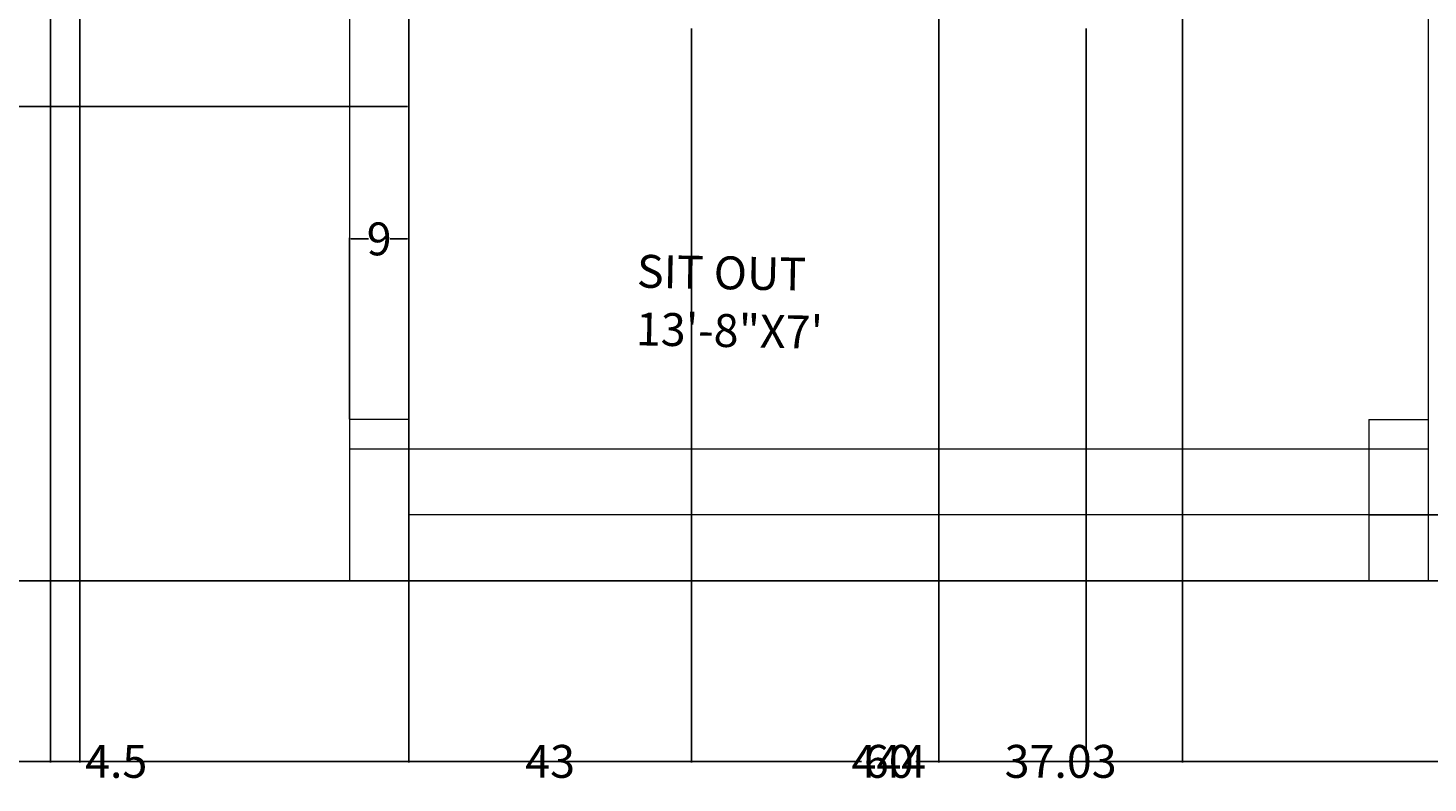
# Model space of a CAD drawing. Units: inches. Extents: x 2807 to 3326, y 2005 to 2580.
# Tile 2 of 12: x 2936 to 3149, y 2005 to 2120. Entities that reach past the tile are written whole.
import ezdxf

# ---------------------------------------------------------------- set-up
doc = ezdxf.new("R2010")
doc.units = ezdxf.units.IN
doc.header["$LTSCALE"] = 0.4
for name, color, linetype, lineweight in [('A-ANNO-DIMS', 2, 'Continuous', 18), ('A-AREA-IDEN', 5, 'Continuous', 18), ('A-FLOR-STRS', 233, 'Continuous', 18)]:
    doc.layers.add(name, color=color, linetype=linetype, lineweight=lineweight)
doc.styles.get("Standard").update_dxf_attribs({"font": 'txt', "height": 5})
doc.dimstyles.get("Standard").update_dxf_attribs({"dimtxt": 0.18, "dimasz": 0.18, "dimexe": 0.18, "dimexo": 0.0625, "dimgap": 0.09, "dimtad": 0, "dimtih": 1, "dimtoh": 1, "dimdec": 4, "dimzin": 0, "dimdsep": 46, "dimtxsty": 'Standard', "dimcen": 0.09, "dimadec": 0, "dimazin": 0, "dimtfac": 1, "dimtdec": 4, "dimtofl": 0, "dimtmove": 0, "dimatfit": 3, "dimfxl": 1, "dimtolj": 1, "dimtzin": 0, "dimarcsym": 0})

# ---------------------------------------------------------------- blocks, each defined once
blk = doc.blocks.new('*D31')
at = {"layer": 'A-ANNO-DIMS', "color": 0, "lineweight": -2, "ltscale": 0.4, "transparency": 16777216}
for p, q in [((2844.57, 2135.51), (2844.57, 2008.45)), ((3288.57, 2135.51), (3288.57, 2008.45)), ((2844.75, 2008.63), (3059.93, 2008.63)), ((3288.39, 2008.63), (3073.2, 2008.63))]:
    blk.add_line(p, q, dxfattribs=at)
at = {"layer": 'A-ANNO-DIMS', "color": 0, "ltscale": 0.4, "transparency": 16777216}
for points in [[(2844.75, 2008.66), (2844.75, 2008.6), (2844.57, 2008.63)], [(3288.39, 2008.66), (3288.39, 2008.6), (3288.57, 2008.63)]]:
    blk.add_solid(points, dxfattribs=at)
at = {"layer": 'Defpoints', "color": 0, "ltscale": 0.4, "transparency": 16777216}
for p in [(2844.57, 2135.58), (3288.57, 2135.58), (3288.57, 2008.63)]:
    blk.add_point(p, dxfattribs=at)
at = {"layer": 'A-ANNO-DIMS', "color": 0, "ltscale": 0.4, "transparency": 16777216, "insert": (3066.57, 2008.63), "char_height": 5, "attachment_point": 5}
blk.add_mtext('\\A1;444', dxfattribs=at)
blk = doc.blocks.new('*D33')
at = {"layer": 'A-ANNO-DIMS', "color": 0, "lineweight": -2, "ltscale": 0.4, "transparency": 16777216}
for p, q in [((2844.504691, 2135.576496), (2816.937191, 2135.576496)), ((2817.117191, 2135.396496), (2817.117191, 2088.416496)), ((2817.117191, 2036.256496), (2817.117191, 2083.236496)), ((2984.504691, 2036.076496), (2816.937191, 2036.076496))]:
    blk.add_line(p, q, dxfattribs=at)
at = {"layer": 'A-ANNO-DIMS', "color": 0, "ltscale": 0.4, "transparency": 16777216}
for points in [[(2817.087191, 2135.396496), (2817.147191, 2135.396496), (2817.117191, 2135.576496)], [(2817.087191, 2036.256496), (2817.147191, 2036.256496), (2817.117191, 2036.076496)]]:
    blk.add_solid(points, dxfattribs=at)
at = {"layer": 'Defpoints', "color": 0, "ltscale": 0.4, "transparency": 16777216}
for p in [(2817.117191, 2135.576496), (2844.567191, 2135.576496), (2984.567191, 2036.076496)]:
    blk.add_point(p, dxfattribs=at)
at = {"layer": 'A-ANNO-DIMS', "color": 0, "ltscale": 0.4, "transparency": 16777216, "insert": (2817.117191, 2085.826496), "char_height": 5, "attachment_point": 5}
blk.add_mtext('\\A1;99.5', dxfattribs=at)
blk = doc.blocks.new('*D34')
at = {"layer": 'A-ANNO-DIMS', "color": 0, "lineweight": -2, "ltscale": 0.4, "transparency": 16777216}
for p, q in [((2984.57, 2060.64), (2984.57, 2088.21)), ((2984.75, 2088.03), (2987.43, 2088.03)), ((2993.39, 2088.03), (2990.7, 2088.03)), ((2993.57, 2060.64), (2993.57, 2088.21))]:
    blk.add_line(p, q, dxfattribs=at)
at = {"layer": 'A-ANNO-DIMS', "color": 0, "ltscale": 0.4, "transparency": 16777216}
for points in [[(2984.75, 2088.06), (2984.75, 2088), (2984.57, 2088.03)], [(2993.39, 2088.06), (2993.39, 2088), (2993.57, 2088.03)]]:
    blk.add_solid(points, dxfattribs=at)
at = {"layer": 'Defpoints', "color": 0, "ltscale": 0.4, "transparency": 16777216}
for p in [(2993.57, 2088.03), (2984.57, 2060.58), (2993.57, 2060.58)]:
    blk.add_point(p, dxfattribs=at)
at = {"layer": 'A-ANNO-DIMS', "color": 0, "ltscale": 0.4, "transparency": 16777216, "insert": (2989.07, 2088.03), "char_height": 5, "attachment_point": 5}
blk.add_mtext('\\A1;9', dxfattribs=at)
blk = doc.blocks.new('*D35')
at = {"layer": 'A-ANNO-DIMS', "color": 0, "lineweight": -2, "ltscale": 0.4, "transparency": 16777216}
for p, q in [((2844.57, 2135.51), (2844.57, 2107.95)), ((2993.57, 2135.51), (2993.57, 2107.95)), ((2844.75, 2108.13), (2913.14, 2108.13)), ((2993.39, 2108.13), (2924.99, 2108.13))]:
    blk.add_line(p, q, dxfattribs=at)
at = {"layer": 'A-ANNO-DIMS', "color": 0, "ltscale": 0.4, "transparency": 16777216}
for points in [[(2844.75, 2108.16), (2844.75, 2108.1), (2844.57, 2108.13)], [(2993.39, 2108.16), (2993.39, 2108.1), (2993.57, 2108.13)]]:
    blk.add_solid(points, dxfattribs=at)
at = {"layer": 'Defpoints', "color": 0, "ltscale": 0.4, "transparency": 16777216}
for p in [(2844.57, 2135.58), (2993.57, 2135.58), (2844.57, 2108.13)]:
    blk.add_point(p, dxfattribs=at)
at = {"layer": 'A-ANNO-DIMS', "color": 0, "ltscale": 0.4, "transparency": 16777216, "insert": (2919.07, 2108.13), "char_height": 5, "attachment_point": 5}
blk.add_mtext('\\A1;149', dxfattribs=at)
blk = doc.blocks.new('*D39')
at = {"layer": 'A-ANNO-DIMS', "color": 0, "lineweight": -2, "ltscale": 0.4, "transparency": 16777216}
for p, q in [((2993.57, 2120.01), (2993.57, 2008.45)), ((3036.57, 2120.01), (3036.57, 2008.45)), ((2993.75, 2008.63), (3010.93, 2008.63)), ((3036.39, 2008.63), (3019.2, 2008.63))]:
    blk.add_line(p, q, dxfattribs=at)
at = {"layer": 'A-ANNO-DIMS', "color": 0, "ltscale": 0.4, "transparency": 16777216}
for points in [[(2993.75, 2008.66), (2993.75, 2008.6), (2993.57, 2008.63)], [(3036.39, 2008.66), (3036.39, 2008.6), (3036.57, 2008.63)]]:
    blk.add_solid(points, dxfattribs=at)
at = {"layer": 'Defpoints', "color": 0, "ltscale": 0.4, "transparency": 16777216}
for p in [(2993.57, 2120.08), (3036.57, 2120.08), (3036.57, 2008.63)]:
    blk.add_point(p, dxfattribs=at)
at = {"layer": 'A-ANNO-DIMS', "color": 0, "ltscale": 0.4, "transparency": 16777216, "insert": (3015.07, 2008.63), "char_height": 5, "attachment_point": 5}
blk.add_mtext('\\A1;43', dxfattribs=at)
blk = doc.blocks.new('*D40')
at = {"layer": 'A-ANNO-DIMS', "color": 0, "lineweight": -2, "ltscale": 0.4, "transparency": 16777216}
for p, q in [((3036.57, 2120.01), (3036.57, 2008.45)), ((3096.57, 2120.01), (3096.57, 2008.45)), ((3036.75, 2008.63), (3062.43, 2008.63)), ((3096.39, 2008.63), (3070.7, 2008.63))]:
    blk.add_line(p, q, dxfattribs=at)
at = {"layer": 'A-ANNO-DIMS', "color": 0, "ltscale": 0.4, "transparency": 16777216}
for points in [[(3036.75, 2008.66), (3036.75, 2008.6), (3036.57, 2008.63)], [(3096.39, 2008.66), (3096.39, 2008.6), (3096.57, 2008.63)]]:
    blk.add_solid(points, dxfattribs=at)
at = {"layer": 'Defpoints', "color": 0, "ltscale": 0.4, "transparency": 16777216}
for p in [(3036.57, 2120.08), (3096.57, 2120.08), (3096.57, 2008.63)]:
    blk.add_point(p, dxfattribs=at)
at = {"layer": 'A-ANNO-DIMS', "color": 0, "ltscale": 0.4, "transparency": 16777216, "insert": (3066.57, 2008.63), "char_height": 5, "attachment_point": 5}
blk.add_mtext('\\A1;60', dxfattribs=at)
blk = doc.blocks.new('*D62')
at = {"layer": 'A-ANNO-DIMS', "color": 0, "lineweight": -2, "ltscale": 0.4, "transparency": 16777216}
for p, q in [((3074.18, 2179.21), (3074.18, 2008.45)), ((3111.21, 2179.53), (3111.21, 2008.45)), ((3074.36, 2008.63), (3082.61, 2008.63)), ((3111.03, 2008.63), (3102.79, 2008.63))]:
    blk.add_line(p, q, dxfattribs=at)
at = {"layer": 'A-ANNO-DIMS', "color": 0, "ltscale": 0.4, "transparency": 16777216}
for points in [[(3074.36, 2008.66), (3074.36, 2008.6), (3074.18, 2008.63)], [(3111.03, 2008.66), (3111.03, 2008.6), (3111.21, 2008.63)]]:
    blk.add_solid(points, dxfattribs=at)
at = {"layer": 'Defpoints', "color": 0, "ltscale": 0.4, "transparency": 16777216}
for p in [(3074.18, 2179.27), (3111.21, 2179.59), (3111.21, 2008.63)]:
    blk.add_point(p, dxfattribs=at)
at = {"layer": 'A-ANNO-DIMS', "color": 0, "ltscale": 0.4, "transparency": 16777216, "insert": (3092.7, 2008.63), "char_height": 5, "attachment_point": 5}
blk.add_mtext('\\A1;37.03', dxfattribs=at)
blk = doc.blocks.new('*D69')
at = {"layer": 'A-ANNO-DIMS', "color": 0, "lineweight": -2, "ltscale": 0.4, "transparency": 16777216}
for p, q in [((2939.07, 2380.01), (2939.07, 2008.45)), ((2943.57, 2380.01), (2943.57, 2008.45)), ((2939.25, 2008.63), (2943.39, 2008.63)), ((2943.57, 2008.63), (2943.75, 2008.63))]:
    blk.add_line(p, q, dxfattribs=at)
at = {"layer": 'A-ANNO-DIMS', "color": 0, "ltscale": 0.4, "transparency": 16777216}
for points in [[(2939.25, 2008.66), (2939.25, 2008.6), (2939.07, 2008.63)], [(2943.39, 2008.66), (2943.39, 2008.6), (2943.57, 2008.63)]]:
    blk.add_solid(points, dxfattribs=at)
at = {"layer": 'Defpoints', "color": 0, "ltscale": 0.4, "transparency": 16777216}
for p in [(2939.07, 2380.08), (2943.57, 2380.08), (2943.57, 2008.63)]:
    blk.add_point(p, dxfattribs=at)
at = {"layer": 'A-ANNO-DIMS', "color": 0, "ltscale": 0.4, "transparency": 16777216, "insert": (2949.08, 2008.63), "char_height": 5, "attachment_point": 5}
blk.add_mtext('\\A1;4.5', dxfattribs=at)
blk = doc.blocks.new('*D73')
at = {"layer": 'A-ANNO-DIMS', "color": 0, "lineweight": -2, "ltscale": 0.4, "transparency": 16777216}
for p, q in [((3139.629691, 2046.076496), (3167.197191, 2046.076496)), ((3167.017191, 2045.896496), (3167.017191, 2043.666496)), ((3167.017191, 2036.256496), (3167.017191, 2038.486496)), ((3139.629691, 2036.076496), (3167.197191, 2036.076496))]:
    blk.add_line(p, q, dxfattribs=at)
at = {"layer": 'A-ANNO-DIMS', "color": 0, "ltscale": 0.4, "transparency": 16777216}
for points in [[(3166.987191, 2045.896496), (3167.047191, 2045.896496), (3167.017191, 2046.076496)], [(3166.987191, 2036.256496), (3167.047191, 2036.256496), (3167.017191, 2036.076496)]]:
    blk.add_solid(points, dxfattribs=at)
at = {"layer": 'Defpoints', "color": 0, "ltscale": 0.4, "transparency": 16777216}
for p in [(3139.567191, 2046.076496), (3139.567191, 2036.076496), (3167.017191, 2036.076496)]:
    blk.add_point(p, dxfattribs=at)
at = {"layer": 'A-ANNO-DIMS', "color": 0, "ltscale": 0.4, "transparency": 16777216, "insert": (3167.017191, 2041.076496), "char_height": 5, "attachment_point": 5}
blk.add_mtext('\\A1;10', dxfattribs=at)

msp = doc.modelspace()

# ---------------------------------------------------------------- linework, layer by layer
at = {"layer": 'A-FLOR-STRS'}
for p, q in [((2984.5672, 2144.5765), (2984.5672, 2036.0765)), ((3148.5672, 2144.5765), (3148.5672, 2036.0765)), ((2993.5672, 2060.5765), (2984.5672, 2060.5765)), ((2993.5672, 2060.5765), (2993.5672, 2036.0765)), ((3139.5672, 2060.5765), (3139.5672, 2036.0765)), ((3139.5672, 2060.5765), (3148.5672, 2060.5765)), ((3148.5672, 2056.0765), (2984.5672, 2056.0765)), ((3139.5672, 2046.0765), (2993.5672, 2046.0765)), ((3148.5672, 2036.0765), (2984.5672, 2036.0765)), ((2984.5672, 2036.0765), (3148.5672, 2036.0765))]:
    msp.add_line(p, q, dxfattribs=at)

# ---------------------------------------------------------------- texts
at = {"layer": 'A-AREA-IDEN', "ltscale": 0.4}
for s, p in [('SIT OUT', (3028.2313, 2080.6324)), ('13\'-8"X7\'', (3028.068, 2071.86))]:
    msp.add_text(s, height=5, rotation=358.933415, dxfattribs=at).set_placement(p)

# ---------------------------------------------------------------- dimensions: what is measured, and where the dimension line sits
at = {"layer": 'A-ANNO-DIMS', "ltscale": 0.4}
for base, p1, p2, override, picture, middle in [((2943.5672, 2008.6265), (2939.0672, 2380.0765), (2943.5672, 2380.0765), {"dimdec": 1, "dimlfac": 1, "dimrnd": 0, "dimzin": 0, "dimdsep": 46, "dimlunit": 2}, '*D69', (2949.0753, 2008.6265)), ((3111.2129, 2008.6265), (3074.1849, 2179.2711), (3111.2129, 2179.5939), {"dimdec": 2, "dimlfac": 1, "dimrnd": 0, "dimzin": 0, "dimdsep": 46, "dimlunit": 2}, '*D62', (3092.6989, 2008.6265)), ((3288.5672, 2008.6265), (2844.5672, 2135.5765), (3288.5672, 2135.5765), {"dimdec": 0, "dimlfac": 1, "dimrnd": 0, "dimzin": 0, "dimdsep": 46, "dimlunit": 2}, '*D31', (3066.5672, 2008.6265)), ((3036.5672, 2008.6265), (2993.5672, 2120.0765), (3036.5672, 2120.0765), {"dimdec": 0, "dimlfac": 1, "dimrnd": 0, "dimzin": 0, "dimdsep": 46, "dimlunit": 2}, '*D39', (3015.0672, 2008.6265)), ((3096.5672, 2008.6265), (3036.5672, 2120.0765), (3096.5672, 2120.0765), {"dimdec": 0, "dimlfac": 1, "dimrnd": 0, "dimzin": 0, "dimdsep": 46, "dimlunit": 2}, '*D40', (3066.5672, 2008.6265)), ((2993.5672, 2088.0265), (2984.5672, 2060.5765), (2993.5672, 2060.5765), {"dimdec": 0, "dimlfac": 1, "dimrnd": 0, "dimzin": 0, "dimdsep": 46, "dimlunit": 2}, '*D34', (2989.0672, 2088.0265))]:
    dim = msp.add_linear_dim(base=base, p1=p1, p2=p2, dimstyle='Standard', override=override, dxfattribs=at)
    dim.commit()
    dim.dimension.update_dxf_attribs({"geometry": picture, "text_midpoint": middle})
for base, p1, p2, angle, override, picture, middle in [((2817.1172, 2135.5765), (2984.5672, 2036.0765), (2844.5672, 2135.5765), 90, {"dimdec": 1, "dimlfac": 1, "dimrnd": 0, "dimzin": 0, "dimdsep": 46, "dimlunit": 2}, '*D33', (2817.1172, 2085.8265)), ((2844.5672, 2108.1265), (2993.5672, 2135.5765), (2844.5672, 2135.5765), 180, {"dimdec": 0, "dimlfac": 1, "dimrnd": 0, "dimzin": 0, "dimdsep": 46, "dimlunit": 2}, '*D35', (2919.0672, 2108.1265)), ((3167.0172, 2036.0765), (3139.5672, 2046.0765), (3139.5672, 2036.0765), 270, {"dimdec": 0, "dimlfac": 1, "dimrnd": 0, "dimzin": 0, "dimdsep": 46, "dimlunit": 2}, '*D73', (3167.0172, 2041.0765))]:
    dim = msp.add_linear_dim(base=base, p1=p1, p2=p2, angle=angle, dimstyle='Standard', override=override, dxfattribs=at)
    dim.commit()
    dim.dimension.update_dxf_attribs({"geometry": picture, "text_midpoint": middle})

doc.saveas('drawing.dxf')
